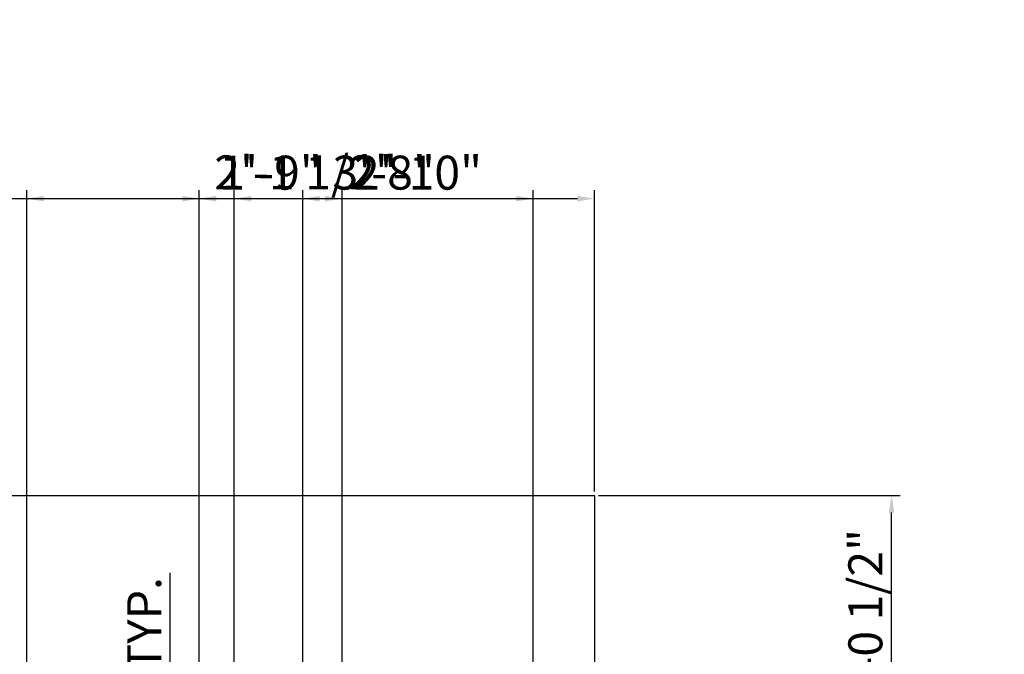
# Model space of a CAD drawing. Units: inches. Extents: x 1804 to 3296, y 909 to 2477.
# Tile 22 of 31: x 2241 to 2386, y 1807 to 1900. Entities that reach past the tile are written whole.
import ezdxf

# ---------------------------------------------------------------- set-up
doc = ezdxf.new("R2010")
doc.units = ezdxf.units.IN
for name, color, linetype, lineweight in [('A-ANNO-DIMS', 2, 'Continuous', 18), ('A-ANNO-TTLB', 156, 'Continuous', 35), ('C-PROP', 7, 'Continuous', 25)]:
    doc.layers.add(name, color=color, linetype=linetype, lineweight=lineweight)
doc.styles.get("Standard").update_dxf_attribs({"font": 'arial.ttf'})
doc.dimstyles.new('ISO-25', dxfattribs={"dimtxt": 5, "dimasz": 2.5, "dimexe": 1.25, "dimexo": 0.625, "dimtad": 1, "dimdec": 0, "dimlunit": 4, "dimtxsty": 'Standard', "dimcen": 2.5, "dimadec": 0, "dimazin": 0, "dimtfac": 1, "dimtdec": 0, "dimtmove": 0, "dimatfit": 3, "dimfxl": 1, "dimarcsym": 0})

# ---------------------------------------------------------------- blocks, each defined once
blk = doc.blocks.new('*D50')
at = {"layer": 'A-ANNO-DIMS', "color": 0, "lineweight": -2, "transparency": 16777216}
for p, q in [((2263.17, 1784.38), (2263.17, 1818.69)), ((2267.38, 1784.38), (2261.92, 1784.38)), ((2263.17, 1759.97), (2263.17, 1781.88)), ((2267.38, 1757.47), (2261.92, 1757.47))]:
    blk.add_line(p, q, dxfattribs=at)
at = {"layer": 'A-ANNO-DIMS', "color": 0, "lineweight": 100, "transparency": 16777216}
for points in [[(2262.75, 1781.88), (2263.59, 1781.88), (2263.17, 1784.38)], [(2262.75, 1759.97), (2263.59, 1759.97), (2263.17, 1757.47)]]:
    blk.add_solid(points, dxfattribs=at)
at = {"layer": 'Defpoints', "color": 0, "lineweight": 100, "transparency": 16777216}
for p in [(2263.17, 1784.38), (2268, 1784.38), (2268, 1757.47)]:
    blk.add_point(p, dxfattribs=at)
at = {"layer": 'A-ANNO-DIMS', "color": 0, "transparency": 16777216, "insert": (2259.99, 1802.79), "char_height": 5, "attachment_point": 5, "rotation": 90}
blk.add_mtext('2\'-3" TYP.', dxfattribs=at)
blk = doc.blocks.new('*D51')
at = {"layer": 'A-ANNO-DIMS', "color": 0, "lineweight": -2, "transparency": 16777216}
for p, q in [((1925.58, 1830.66), (1925.58, 1874.99)), ((2325.54, 1830.66), (2325.54, 1874.99)), ((1928.08, 1873.74), (2323.04, 1873.74))]:
    blk.add_line(p, q, dxfattribs=at)
at = {"layer": 'A-ANNO-DIMS', "color": 0, "lineweight": 100, "transparency": 16777216}
for points in [[(1928.08, 1874.15), (1928.08, 1873.32), (1925.58, 1873.74)], [(2323.04, 1874.15), (2323.04, 1873.32), (2325.54, 1873.74)]]:
    blk.add_solid(points, dxfattribs=at)
at = {"layer": 'Defpoints', "color": 0, "lineweight": 100, "transparency": 16777216}
for p in [(2325.54, 1873.74), (1925.58, 1830.04), (2325.54, 1830.04)]:
    blk.add_point(p, dxfattribs=at)
at = {"layer": 'A-ANNO-DIMS', "color": 0, "transparency": 16777216, "insert": (2125.56, 1876.92), "char_height": 5, "attachment_point": 5}
blk.add_mtext('33\'-4"', dxfattribs=at)
blk = doc.blocks.new('*D55')
at = {"layer": 'A-ANNO-DIMS', "color": 0, "lineweight": -2, "transparency": 16777216}
for p, q in [((2326.16, 1830.04), (2370.49, 1830.04)), ((2369.24, 1795.88), (2369.24, 1827.54)), ((2326.16, 1793.38), (2370.49, 1793.38))]:
    blk.add_line(p, q, dxfattribs=at)
at = {"layer": 'A-ANNO-DIMS', "color": 0, "lineweight": 100, "transparency": 16777216}
for points in [[(2368.82, 1827.54), (2369.65, 1827.54), (2369.24, 1830.04)], [(2368.82, 1795.88), (2369.65, 1795.88), (2369.24, 1793.38)]]:
    blk.add_solid(points, dxfattribs=at)
at = {"layer": 'Defpoints', "color": 0, "lineweight": 100, "transparency": 16777216}
for p in [(2325.54, 1830.04), (2369.24, 1830.04), (2325.54, 1793.38)]:
    blk.add_point(p, dxfattribs=at)
at = {"layer": 'A-ANNO-DIMS', "color": 0, "transparency": 16777216, "insert": (2366.03, 1811.71), "char_height": 5, "attachment_point": 5, "rotation": 90}
blk.add_mtext('3\'-0 1/2"', dxfattribs=at)
blk = doc.blocks.new('*D65')
at = {"layer": 'A-ANNO-DIMS', "color": 0, "lineweight": -2, "transparency": 16777216}
for p, q in [((2282.65, 1466.57), (2282.65, 1874.99)), ((2316.54, 1466.57), (2316.54, 1874.99)), ((2285.15, 1873.74), (2314.04, 1873.74))]:
    blk.add_line(p, q, dxfattribs=at)
at = {"layer": 'A-ANNO-DIMS', "color": 0, "lineweight": 100, "transparency": 16777216}
for points in [[(2285.15, 1874.15), (2285.15, 1873.32), (2282.65, 1873.74)], [(2314.04, 1874.15), (2314.04, 1873.32), (2316.54, 1873.74)]]:
    blk.add_solid(points, dxfattribs=at)
at = {"layer": 'Defpoints', "color": 0, "lineweight": 100, "transparency": 16777216}
for p in [(2316.54, 1873.74), (2282.65, 1465.94), (2316.54, 1465.94)]:
    blk.add_point(p, dxfattribs=at)
at = {"layer": 'A-ANNO-DIMS', "color": 0, "transparency": 16777216, "insert": (2299.6, 1876.91), "char_height": 5, "attachment_point": 5}
blk.add_mtext('2\'-10"', dxfattribs=at)
blk = doc.blocks.new('*D67')
at = {"layer": 'A-ANNO-DIMS', "color": 0, "lineweight": -2, "transparency": 16777216}
for p, q in [((2267.43, 1587.05), (2267.43, 1874.99)), ((2288.43, 1587.05), (2288.43, 1874.99)), ((2269.93, 1873.74), (2285.93, 1873.74))]:
    blk.add_line(p, q, dxfattribs=at)
at = {"layer": 'A-ANNO-DIMS', "color": 0, "lineweight": 100, "transparency": 16777216}
for points in [[(2269.93, 1874.15), (2269.93, 1873.32), (2267.43, 1873.74)], [(2285.93, 1874.15), (2285.93, 1873.32), (2288.43, 1873.74)]]:
    blk.add_solid(points, dxfattribs=at)
at = {"layer": 'Defpoints', "color": 0, "lineweight": 100, "transparency": 16777216}
for p in [(2288.43, 1873.74), (2267.43, 1586.42), (2288.43, 1586.42)]:
    blk.add_point(p, dxfattribs=at)
at = {"layer": 'A-ANNO-DIMS', "color": 0, "transparency": 16777216, "insert": (2277.93, 1876.91), "char_height": 5, "attachment_point": 5}
blk.add_mtext('1\'-9"', dxfattribs=at)
blk = doc.blocks.new('*D68')
at = {"layer": 'A-ANNO-DIMS', "color": 0, "lineweight": -2, "transparency": 16777216}
for p, q in [((2242.06, 1587.05), (2242.06, 1874.99)), ((2267.43, 1587.05), (2267.43, 1874.99)), ((2244.56, 1873.74), (2264.93, 1873.74)), ((2267.43, 1873.74), (2296.2, 1873.74))]:
    blk.add_line(p, q, dxfattribs=at)
at = {"layer": 'A-ANNO-DIMS', "color": 0, "lineweight": 100, "transparency": 16777216}
for points in [[(2244.56, 1874.15), (2244.56, 1873.32), (2242.06, 1873.74)], [(2264.93, 1874.15), (2264.93, 1873.32), (2267.43, 1873.74)]]:
    blk.add_solid(points, dxfattribs=at)
at = {"layer": 'Defpoints', "color": 0, "lineweight": 100, "transparency": 16777216}
for p in [(2267.43, 1873.74), (2242.06, 1586.42), (2267.43, 1586.42)]:
    blk.add_point(p, dxfattribs=at)
at = {"layer": 'A-ANNO-DIMS', "color": 0, "transparency": 16777216, "insert": (2283.07, 1876.95), "char_height": 5, "attachment_point": 5}
blk.add_mtext('2\'-1 1/2"', dxfattribs=at)
blk = doc.blocks.new('*D73')
at = {"layer": 'A-ANNO-DIMS', "color": 0, "lineweight": -2, "transparency": 16777216}
for p, q in [((2272.59, 1272.26), (2272.59, 1874.99)), ((2316.54, 1272.26), (2316.54, 1874.99)), ((2275.09, 1873.74), (2314.04, 1873.74))]:
    blk.add_line(p, q, dxfattribs=at)
at = {"layer": 'A-ANNO-DIMS', "color": 0, "lineweight": 100, "transparency": 16777216}
for points in [[(2275.09, 1874.15), (2275.09, 1873.32), (2272.59, 1873.74)], [(2314.04, 1874.15), (2314.04, 1873.32), (2316.54, 1873.74)]]:
    blk.add_solid(points, dxfattribs=at)
at = {"layer": 'Defpoints', "color": 0, "lineweight": 100, "transparency": 16777216}
for p in [(2316.54, 1873.74), (2272.59, 1271.63), (2316.54, 1271.63)]:
    blk.add_point(p, dxfattribs=at)
at = {"layer": 'A-ANNO-DIMS', "color": 0, "transparency": 16777216, "insert": (2294.56, 1876.92), "char_height": 5, "attachment_point": 5}
blk.add_mtext('3\'-8"', dxfattribs=at)

msp = doc.modelspace()

# ---------------------------------------------------------------- hatches: boundary and pattern name
at = {"layer": 'A-ANNO-TTLB'}
h = msp.add_hatch(color=256, dxfattribs=at)
h.dxf.hatch_style = 1
h.paths.add_polyline_path([(3294.53, 2476.54), (1803.79, 2476.54), (1805.43, 909.47), (3296.17, 909.47)])
h.paths.add_polyline_path([(1811, 914.33), (1812.79, 2467.54), (3285.53, 2467.54), (3283.74, 914.33)], flags=16)
h.paths.add_polyline_path([(1925.58, 1062.77), (1925.58, 1138.07), (1925.58, 1539.88), (1925.58, 1793.38), (1925.58, 1830.04), (2325.54, 1830.04), (2325.54, 1793.38), (2325.54, 1586.42), (2325.54, 1138.07), (2325.54, 1062.77)], flags=0)
h.paths.add_polyline_path([(1997.22, 1029.4), (2008.85, 1037.96), (2008.85, 1020.84)], flags=0)
h.paths.add_polyline_path([(1934.58, 1138.07), (1934.58, 1147.07), (2078.77, 1147.07), (2078.77, 1138.07), (2060.94, 1138.07)], flags=0)
h.paths.add_polyline_path([(1944.35, 1138.07), (1944.35, 1147.07), (2056.05, 1147.07), (2056.05, 1138.07)], flags=0)
h.paths.add_polyline_path([(2222.24, 1037.96), (2233.87, 1029.4), (2222.24, 1020.84)], flags=0)
h.paths.add_polyline_path([(2061.94, 1139.07), (2061.94, 1146.07), (2077.77, 1146.07), (2077.77, 1139.07)], flags=0)
h.paths.add_polyline_path([(2149.58, 1138.07), (2149.58, 1269.44), (2158.58, 1269.44), (2158.58, 1326.69), (2149.58, 1326.69), (2149.58, 1340.94), (2139.6, 1340.94), (2139.6, 1434.25), (2149.58, 1434.25), (2149.58, 1447.36), (2158.58, 1447.36), (2158.58, 1423.87), (2158.58, 1408.06), (2198.46, 1408.06), (2198.46, 1412.56), (2282.65, 1412.56), (2282.65, 1465.94), (2316.54, 1465.94), (2316.54, 1590.92), (2192.86, 1590.92), (2192.86, 1595.3), (2291.17, 1595.3), (2291.17, 1590.92), (2316.54, 1590.92), (2316.54, 1784.38), (2300.24, 1784.38), (2300.24, 1757.47), (2268, 1757.47), (2268, 1681.04), (2180.87, 1681.04), (2180.87, 1757.47), (2148.63, 1757.47), (2148.63, 1784.38), (2119.08, 1784.38), (2119.08, 1585.58), (2114.58, 1585.58), (2114.58, 1784.38), (2064.11, 1784.38), (2046.28, 1784.38), (2046.28, 1760.38), (1958.58, 1760.38), (1958.58, 1664.38), (1934.58, 1664.38), (1934.58, 1784.38), (1934.58, 1793.38), (2046.28, 1793.38), (2064.11, 1793.38), (2119.08, 1793.38), (2230.78, 1793.38), (2230.78, 1784.38), (2268, 1784.38), (2300.24, 1784.38), (2316.54, 1784.38), (2316.54, 1590.92), (2316.54, 1373.73), (2316.54, 1138.07)], flags=0)
h.paths.add_polyline_path([(2209.19, 1166.63), (2209.19, 1175.63), (2158.58, 1175.63), (2209.19, 1223.63), (2209.19, 1231.63), (2183.88, 1231.63), (2183.88, 1301.66), (2242.59, 1301.66), (2242.59, 1326.69), (2316.54, 1326.69), (2272.59, 1271.63), (2272.59, 1223.63), (2316.54, 1175.63), (2272.59, 1175.63), (2272.59, 1166.63)], flags=0)
h.paths.add_polyline_path([(1947.77, 1345.22), (1947.77, 1457.48), (1991.2, 1457.48), (1991.2, 1451.7), (1991.2, 1352.18), (1991.2, 1345.22)], flags=0)
h.paths.add_polyline_path([(2209.19, 1271.63), (2262.59, 1271.63), (2262.59, 1311.85), (2272.59, 1301.66), (2272.59, 1271.63), (2269.92, 1269.63), (2270.59, 1269.63), (2270.59, 1225.63), (2211.19, 1225.63), (2211.19, 1269.63), (2211.86, 1269.63)], flags=0)
h.paths.add_polyline_path([(2000.34, 1378.21), (2000.34, 1429.71), (2025.22, 1429.71), (2025.22, 1378.21)], flags=0)
h.paths.add_polyline_path([(2001.34, 1379.21), (2001.34, 1428.71), (2024.22, 1428.71), (2024.22, 1379.21)], flags=0)
h.paths.add_polyline_path([(2012.34, 1390.21), (2012.34, 1417.71), (2013.22, 1417.71), (2013.22, 1390.21)], flags=0)
h.paths.add_polyline_path([(2237.56, 1331.19), (2237.56, 1340.18), (2238.62, 1340.18), (2238.62, 1386.84), (2241.04, 1386.84), (2242.06, 1386.84), (2242.06, 1408.06), (2316.54, 1331.19)], flags=0)
h.paths.add_polyline_path([(1953.73, 1464.35), (1953.73, 1498.59), (1981.74, 1498.59), (1981.74, 1464.35)], flags=0)
h.paths.add_polyline_path([(1987.63, 1462.08), (1987.63, 1500.95), (2104.07, 1500.95), (2104.07, 1462.08), (2099.27, 1462.08), (1993.6, 1462.08)], flags=0)
h.paths.add_polyline_path([(1956.06, 1481.47, -1), (1979.41, 1481.47, -1)], flags=0)
edge = h.paths.add_edge_path(flags=0)
edge.add_ellipse((2299.53, 1438.37), major_axis=(0.31, 21.36), ratio=0.670333, start_angle=0, end_angle=360)
h.paths.add_polyline_path([(2297.39, 1438.37, -1), (2301.67, 1438.37, -1)], flags=0)
h.paths.add_polyline_path([(2591.54, 1163.23), (2591.54, 1179.38), (2591.54, 1379.68), (2591.54, 1395.84), (2734.5, 1395.84), (2734.5, 1379.68), (2734.5, 1179.38), (2734.5, 1163.23)], flags=0)
h.paths.add_polyline_path([(2592.54, 1164.23), (2592.54, 1166.23), (2733.5, 1166.23), (2733.5, 1164.23)], flags=0)
h.paths.add_polyline_path([(2592.54, 1180.38), (2592.54, 1378.68), (2733.5, 1378.68), (2733.5, 1180.38)], flags=0)
h.paths.add_polyline_path([(2593.54, 1181.38), (2593.54, 1377.68), (2732.5, 1377.68), (2732.5, 1181.38)], flags=0)
h.paths.add_polyline_path([(2594.54, 1182.38), (2594.54, 1376.68), (2731.5, 1376.68), (2731.5, 1182.38)], flags=0)
h.paths.add_polyline_path([(1936.95, 1697.46), (1936.95, 1736.46), (1955.41, 1736.46), (1955.41, 1697.46)], flags=0)
h.paths.add_polyline_path([(1938.48, 1718.36), (1938.48, 1734.92), (1953.65, 1734.92), (1953.65, 1718.36)], flags=0)
h.paths.add_polyline_path([(1944.75, 1726.64, -1), (1947.37, 1726.64, -1)], flags=0)
h.paths.add_polyline_path([(2592.54, 1394.84), (2733.5, 1394.84), (2733.5, 1392.84), (2592.54, 1392.84)], flags=0)
h.paths.add_polyline_path([(1976.61, 1762.5), (1976.61, 1781.44), (2012.79, 1781.44), (2012.79, 1762.5)], flags=0)
h.paths.add_polyline_path([(1979.57, 1771.97, -1), (1991.39, 1771.97, -1)], flags=0)
h.paths.add_polyline_path([(1995.36, 1771.97, -1), (2007.18, 1771.97, -1)], flags=0)
h.paths.add_polyline_path([(2251.51, 1744.53), (2268, 1730.05), (2251.51, 1730.05)], flags=0)
h.paths.add_polyline_path([(2047.28, 1785.38), (2047.28, 1792.38), (2063.11, 1792.38), (2063.11, 1785.38)], flags=0)
h.paths.add_polyline_path([(2155.08, 1770.92, -1), (2174.42, 1770.92, -1)], flags=0)
h.paths.add_polyline_path([(2188.59, 1758.27), (2188.59, 1772.81), (2222.3, 1772.81), (2222.3, 1758.27)], flags=0)
h.paths.add_polyline_path([(2223.97, 1758.27), (2223.97, 1772.81), (2257.68, 1772.81), (2257.68, 1758.27)], flags=0)
h.paths.add_polyline_path([(2274.45, 1770.92, -1), (2293.8, 1770.92, -1)], flags=0)
h.paths.add_polyline_path([(2591.54, 1582.09), (2591.54, 1782.39), (2734.5, 1782.39), (2734.5, 1582.09)], flags=0)
h.paths.add_polyline_path([(2592.54, 1583.09), (2592.54, 1781.39), (2733.5, 1781.39), (2733.5, 1583.09)], flags=0)
h.paths.add_polyline_path([(2593.54, 1584.09), (2593.54, 1780.39), (2732.5, 1780.39), (2732.5, 1584.09)], flags=0)
h.paths.add_polyline_path([(2594.54, 1585.09), (2594.54, 1779.39), (2731.5, 1779.39), (2731.5, 1585.09)], flags=0)
h.paths.add_polyline_path([(1922.17, 1978.79), (1922.17, 2295.08), (1922.17, 2296.08), (2115.67, 2296.08), (2115.67, 2384.31), (2115.67, 2385.31), (2322.12, 2385.31), (2323.12, 2385.31), (2323.12, 1979.79), (2323.12, 1978.79), (1923.17, 1978.79)], flags=0)
h.paths.add_polyline_path([(1922.17, 1978.79), (1922.17, 2051.31), (1922.17, 2214.86), (1922.17, 2296.08), (2115.67, 2296.08), (2115.67, 2385.31), (2323.12, 2385.31), (2323.12, 2280.42), (2323.12, 1978.79), (2115.67, 1978.79)], flags=0)
h.paths.add_polyline_path([(1923.17, 1979.79), (1923.17, 2050.31), (2115.67, 2050.31), (2115.67, 2051.31), (1923.17, 2051.31), (1923.17, 2213.86), (1923.17, 2214.86), (1923.17, 2295.08), (1990.02, 2295.08), (1990.02, 2214.86), (1991.02, 2214.86), (1991.02, 2295.08), (2115.67, 2295.08), (2115.67, 1979.79), (2116.67, 1979.79), (2116.67, 2304.18), (2116.67, 2384.31), (2322.12, 2384.31), (2322.12, 2280.42), (2322.12, 1979.79), (2115.67, 1979.79)], flags=0)
h.paths.add_polyline_path([(2972.46, 1192.5), (2972.46, 1196.92), (2995.47, 1196.92), (2995.47, 1255.47), (2995.09, 1255.47), (2987.42, 1249.39), (2980.08, 1255.47), (2978.05, 1255.47), (2978.05, 1257.24), (2995.47, 1257.24), (2995.47, 1261.58), (3015.37, 1261.58), (3015.37, 1333.28), (3015.37, 1414.4), (3032.82, 1414.4), (3032.82, 1333.28), (3032.82, 1261.58), (3052.66, 1261.58), (3052.66, 1255.47), (3079.86, 1255.47), (3078.72, 1254.57), (3081.47, 1252.29), (3078.56, 1249.99), (3075.81, 1252.26), (3072.57, 1249.69), (3070.36, 1251.52), (3067.67, 1249.39), (3060.34, 1255.47), (3052.66, 1255.47), (3052.66, 1196.92), (3054.58, 1196.92), (3074, 1196.92), (3074, 1192.5), (3052.66, 1192.5), (2995.47, 1192.5)], flags=0)
h.paths.add_polyline_path([(2490.75, 1979.27), (2490.75, 1980.27), (2596.87, 1980.27), (2596.87, 2051.8), (2596.87, 2052.8), (2596.87, 2216.35), (2596.87, 2297.57), (2717.32, 2297.57), (2710.57, 2305.62), (2724.07, 2305.62), (2717.32, 2297.57), (2782.37, 2297.57), (2782.37, 2395.8), (3006.82, 2395.8), (3006.82, 1981.27), (3093.73, 1981.27), (3093.73, 1980.27), (3047.51, 1980.27), (3046.37, 1979.37), (3049.11, 1977.1), (3046.2, 1974.79), (3043.46, 1977.07), (3040.21, 1974.49), (3038, 1976.32), (3035.32, 1974.2), (3027.98, 1980.27), (2871.83, 1980.27), (2871.83, 1981.27), (2791.37, 1981.27), (2791.37, 2050.8), (2597.87, 2050.8), (2597.87, 1980.27), (2597.87, 1979.27), (2546.27, 1979.27), (2545.12, 1978.37), (2547.87, 1976.1), (2544.96, 1973.79), (2542.22, 1976.07), (2538.97, 1973.49), (2536.76, 1975.32), (2534.07, 1973.2), (2526.74, 1979.27)], flags=0)
h.paths.add_polyline_path([(2597.87, 2051.8), (2606.87, 2051.8), (2606.87, 2258.39), (2597.87, 2258.39), (2597.87, 2296.57), (2606.87, 2296.57), (2606.87, 2262.39), (2782.37, 2262.39), (2782.37, 2296.57), (2790.37, 2296.57), (2790.37, 2262.39), (2791.37, 2262.39), (2791.37, 2305.67), (2791.37, 2385.8), (2996.82, 2385.8), (2996.82, 2339.85), (3006.82, 2339.85), (3006.82, 2250.12), (2997.82, 2250.12), (2997.82, 1981.27), (2996.82, 1981.27), (2872.83, 1981.27), (2872.83, 1991.8), (2871.83, 1991.8), (2871.83, 2050.8), (2790.37, 2050.8), (2597.87, 2050.8)], flags=0)
h.paths.add_polyline_path([(2179.93, 2153.92), (2179.93, 2353.97), (2259.98, 2353.97), (2259.98, 2153.92)], flags=0)
h.paths.add_polyline_path([(2180.93, 2154.92), (2180.93, 2352.97), (2258.98, 2352.97), (2258.98, 2154.92)], flags=0)
h.paths.add_polyline_path([(2960.87, 1608.49), (2960.87, 1753.62), (3070.9, 1753.62), (3070.9, 1608.49)], flags=0)
h.paths.add_polyline_path([(2961.87, 1609.49), (2961.87, 1752.62), (3069.9, 1752.62), (3069.9, 1609.49)], flags=0)
h.paths.add_polyline_path([(2962.87, 1610.49), (2962.87, 1751.62), (3068.9, 1751.62), (3068.9, 1610.49)], flags=0)
h.paths.add_polyline_path([(2963.87, 1611.49), (2963.87, 1750.62), (3067.9, 1750.62), (3067.9, 1611.49)], flags=0)
h.paths.add_polyline_path([(2782.37, 2051.8), (2782.37, 2216.32), (2791.37, 2216.32), (2791.37, 2051.8), (2872.83, 2051.8), (2872.83, 2068.56), (2884.67, 2068.56), (2884.67, 2085.33), (2896.51, 2085.33), (2896.51, 2102.09), (2908.36, 2102.09), (2908.36, 2118.85), (2920.2, 2118.85), (2920.2, 2135.62), (2932.05, 2135.62), (2932.05, 2145.3), (2925.08, 2145.3), (2925.08, 2203.2), (2996.82, 2203.2), (2996.82, 2145.3), (2953.82, 2145.3), (2872.83, 2051.8), (2790.37, 2051.8)], flags=0)
h.paths.add_polyline_path([(2717.32, 2238.65), (2710.57, 2246.7), (2724.07, 2246.7)], flags=0)
h.paths.add_polyline_path([(2003.09, 1122.79), (2017.16, 1122.79), (2017.16, 1138.74), (2003.09, 1138.74)], flags=8)
h.paths.add_polyline_path([(2174.76, 1792.72), (2188.83, 1792.72), (2188.83, 1808.66), (2174.76, 1808.66)], flags=8)
h.paths.add_polyline_path([(1987.95, 1792.51), (2002.02, 1792.51), (2002.02, 1808.45), (1987.95, 1808.45)], flags=8)
h.paths.add_polyline_path([(2148.79, 1289.26), (2160.46, 1289.26), (2160.46, 1305.2), (2148.79, 1305.2)], flags=8)
h.paths.add_polyline_path([(2115.36, 1133.57), (2127.04, 1133.57), (2127.04, 1149.51), (2115.36, 1149.51)], flags=8)
h.paths.add_polyline_path([(2237.58, 1421.48), (2249.25, 1421.48), (2249.25, 1437.43), (2237.58, 1437.43)], flags=8)
h.paths.add_polyline_path([(2134.99, 1584.32), (2146.66, 1584.32), (2146.66, 1600.26), (2134.99, 1600.26)], flags=8)
h.paths.add_polyline_path([(2101.95, 1557.31), (2113.62, 1557.31), (2113.62, 1573.25), (2101.95, 1573.25)], flags=8)
h.paths.add_polyline_path([(2937.85, 1156.77), (3120.41, 1156.77), (3120.41, 1185.72), (2937.85, 1185.72)], flags=8)
h.paths.add_polyline_path([(2980.71, 1786.71), (3050.06, 1786.71), (3050.06, 1802.66), (2980.71, 1802.66)], flags=8)
h.paths.add_polyline_path([(2869.28, 1661.96), (2938.62, 1661.96), (2938.62, 1690.8), (2869.28, 1690.8)], flags=8)
h.paths.add_polyline_path([(3092.27, 1674.86), (3161.62, 1674.86), (3161.62, 1690.8), (3092.27, 1690.8)], flags=8)
h.paths.add_polyline_path([(2980.71, 1674.86), (3050.06, 1674.86), (3050.06, 1690.8), (2980.71, 1690.8)], flags=8)
h.paths.add_polyline_path([(2649.07, 1678.23), (2674.53, 1678.23), (2674.53, 1714.76), (2649.07, 1714.76)], flags=8)
h.paths.add_polyline_path([(2530.84, 1981.63), (2549.13, 1981.63), (2549.13, 1997.57), (2530.84, 1997.57)], flags=8)
h.paths.add_polyline_path([(3031.29, 1981.77), (3049.58, 1981.77), (3049.58, 1997.71), (3031.29, 1997.71)], flags=8)
h.paths.add_polyline_path([(2715.38, 1911.9), (2851.54, 1911.9), (2851.54, 1940.85), (2715.38, 1940.85)], flags=8)
h.paths.add_polyline_path([(2015.23, 1927.36), (2205.42, 1927.36), (2205.42, 1956.3), (2015.23, 1956.3)], flags=8)
h.paths.add_polyline_path([(2671.84, 2057.84), (2702.75, 2057.84), (2702.75, 2073.79), (2671.84, 2073.79)], flags=8)
h.paths.add_polyline_path([(2678.5, 2316.52), (2765.26, 2316.52), (2765.26, 2332.46), (2678.5, 2332.46)], flags=8)
h.paths.add_polyline_path([(2678.48, 2271.96), (2736.41, 2271.96), (2736.41, 2287.9), (2678.48, 2287.9)], flags=8)
h.paths.add_polyline_path([(2019.2, 972.79), (2243.21, 972.79), (2243.21, 1001.74), (2019.2, 1001.74)], flags=8)
h.paths.add_polyline_path([(2097.06, 1021.56), (2132.16, 1021.56), (2132.16, 1037.51), (2097.06, 1037.51)], flags=8)
h.paths.add_polyline_path([(2182.47, 1360.48), (2207.35, 1360.48), (2207.35, 1376.42), (2182.47, 1376.42)], flags=8)
h.paths.add_polyline_path([(2261.12, 1361.77), (2295.01, 1361.77), (2295.01, 1377.71), (2261.12, 1377.71)], flags=8)
h.paths.add_polyline_path([(2245.75, 1511.51), (2278.44, 1511.51), (2278.44, 1527.46), (2245.75, 1527.46)], flags=8)
h.paths.add_polyline_path([(1991.16, 1296.29), (2060.51, 1296.29), (2060.51, 1312.23), (1991.16, 1312.23)], flags=8)
h.paths.add_polyline_path([(2187, 1651.35), (2246.71, 1651.35), (2246.71, 1667.29), (2187, 1667.29)], flags=8)
h.paths.add_polyline_path([(1976.49, 1684.81), (2068.63, 1684.81), (2068.63, 1700.76), (1976.49, 1700.76)], flags=8)

# ---------------------------------------------------------------- linework, layer by layer
at = {"layer": 'C-PROP'}
for p, q in [((1925.58, 1830.04), (2325.54, 1830.04)), ((2325.54, 1830.04), (2325.54, 1793.38))]:
    msp.add_line(p, q, dxfattribs=at)

# ---------------------------------------------------------------- dimensions: what is measured, and where the dimension line sits
at = {"layer": 'A-ANNO-DIMS'}
for base, p1, p2, picture, middle in [((2267.43, 1873.74), (2242.06, 1586.42), (2267.43, 1586.42), '*D68', (2283.07, 1876.95)), ((2325.54, 1873.74), (1925.58, 1830.04), (2325.54, 1830.04), '*D51', (2125.56, 1876.92)), ((2288.43, 1873.74), (2267.43, 1586.42), (2288.43, 1586.42), '*D67', (2277.93, 1876.91)), ((2316.5375, 1873.7362), (2272.5886, 1271.6342), (2316.5375, 1271.6342), '*D73', (2294.563, 1876.9158)), ((2316.54, 1873.74), (2282.65, 1465.94), (2316.54, 1465.94), '*D65', (2299.6, 1876.91))]:
    dim = msp.add_linear_dim(base=base, p1=p1, p2=p2, dimstyle='ISO-25', override={"dimdec": 1, "dimlfac": 1, "dimrnd": 0, "dimzin": 1, "dimdsep": 46, "dimlunit": 4, "dimfrac": 2}, dxfattribs=at)
    dim.commit()
    dim.dimension.update_dxf_attribs({"geometry": picture, "text_midpoint": middle})
dim = msp.add_linear_dim(base=(2369.24, 1830.04), p1=(2325.54, 1793.38), p2=(2325.54, 1830.04), angle=90, dimstyle='ISO-25', override={"dimdec": 1, "dimlfac": 1, "dimrnd": 0, "dimzin": 1, "dimdsep": 46, "dimlunit": 4, "dimfrac": 2}, dxfattribs=at)
dim.commit()
dim.dimension.update_dxf_attribs({"geometry": '*D55', "text_midpoint": (2366.03, 1811.71)})
dim = msp.add_linear_dim(base=(2263.17, 1784.38), p1=(2268, 1757.47), p2=(2268, 1784.38), angle=90, text='<> TYP.', dimstyle='ISO-25', override={"dimdec": 1, "dimlfac": 1, "dimrnd": 0, "dimzin": 1, "dimdsep": 46, "dimlunit": 4, "dimfrac": 2}, dxfattribs=at)
dim.commit()
dim.dimension.update_dxf_attribs({"geometry": '*D50', "text_midpoint": (2259.99, 1802.79)})

doc.saveas('drawing.dxf')
